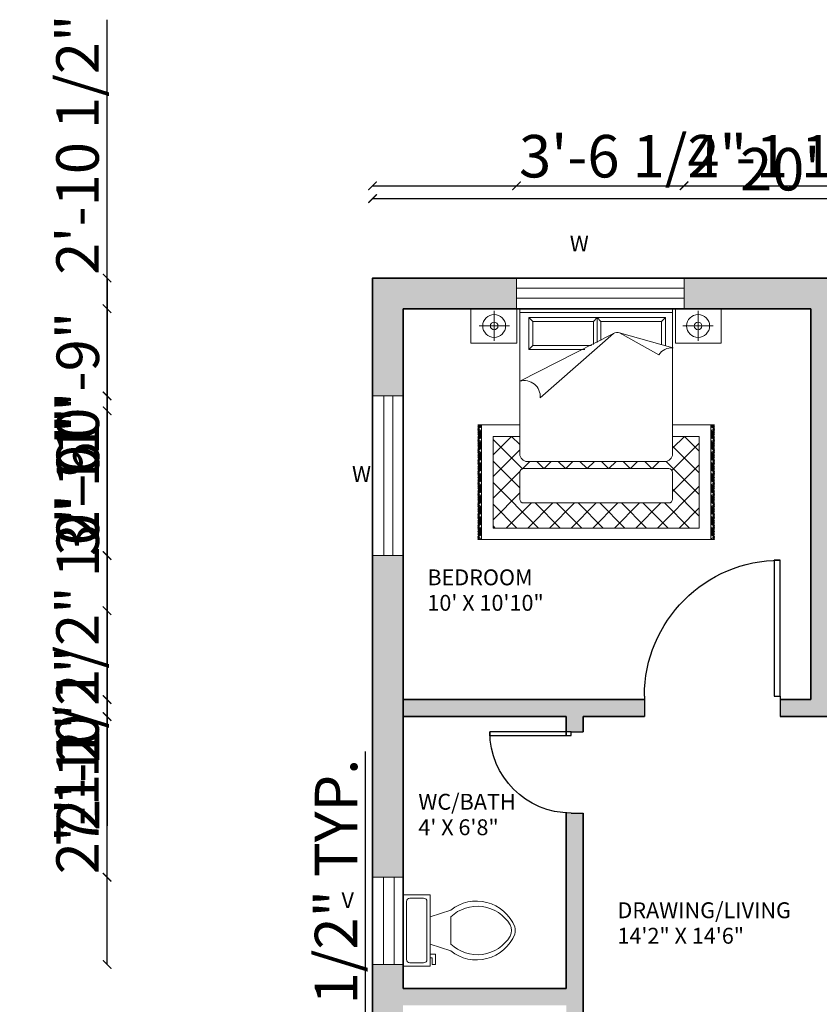
# Model space of a CAD drawing. Units: inches. Extents: x 1750 to 7466, y 1409 to 2004.
# Tile 3 of 5: x 1750 to 1986, y 1715 to 2004. Entities that reach past the tile are written whole.
import ezdxf

# ---------------------------------------------------------------- set-up
doc = ezdxf.new("R2010")
doc.units = ezdxf.units.IN
for name, color, linetype, lineweight in [('A-ANNO-DIMS', 2, 'Continuous', 18), ('A-ANNO-TEXT', 7, 'Continuous', 18), ('A-AREA-IDEN', 7, 'Continuous', 18), ('A-DOOR', 3, 'Continuous', 25), ('A-FLOR-FIXT', 9, 'Continuous', 18), ('A-WALL', 7, 'Continuous', 35), ('BEDS', 15, 'Continuous', 18), ('WINDOW', 4, 'Continuous', 18)]:
    doc.layers.add(name, color=color, linetype=linetype, lineweight=lineweight)
doc.layers.add('A-WALL-PATT', color=18, linetype='Continuous', lineweight=13, true_color=0x000000)
doc.styles.get("Standard").update_dxf_attribs({"font": 'arial.ttf'})
doc.dimstyles.new('ISO-25', dxfattribs={"dimtxt": 12.5, "dimasz": 2.5, "dimexe": 1.25, "dimexo": 0.625, "dimtad": 1, "dimdec": 0, "dimlunit": 4, "dimtxsty": 'Standard', "dimblk": 'ARCHTICK', "dimcen": 2.5, "dimse1": 1, "dimse2": 1, "dimclrd": 2, "dimadec": 0, "dimazin": 0, "dimtfac": 1, "dimtdec": 0, "dimtmove": 0, "dimatfit": 3, "dimfxl": 1, "dimarcsym": 0})

# ---------------------------------------------------------------- blocks, each defined once
blk = doc.blocks.new('A$C4CB008C5')
for p, q in [((0, 3.019), (0.6, 3.019)), ((0, 2.569), (0, 3.019)), ((0.304, 2.6), (0.304, 2.992)), ((0.6, 3.019), (0.6, 2.569)), ((0.64, 1.121), (0.64, 3.021)), ((0.64, 3.021), (2.64, 3.021)), ((0.64, 2.971), (2.64, 2.971)), ((2.64, 3.021), (2.64, 1.121)), ((3.279, 3.019), (2.679, 3.019)), ((2.679, 3.019), (2.679, 2.569)), ((2.975, 2.6), (2.975, 2.992)), ((3.279, 2.569), (3.279, 3.019)), ((0.759, 2.905), (2.547, 2.905)), ((0.759, 2.489), (0.759, 2.905)), ((0.759, 2.905), (0.809, 2.855)), ((0.809, 2.855), (1.603, 2.855)), ((0.809, 2.539), (0.809, 2.855)), ((1.603, 2.855), (1.653, 2.905)), ((1.603, 2.855), (1.603, 2.551)), ((1.653, 2.905), (1.653, 2.579)), ((1.653, 2.905), (1.703, 2.855)), ((1.703, 2.855), (1.703, 2.607)), ((1.703, 2.855), (2.497, 2.855)), ((2.497, 2.855), (2.547, 2.905)), ((2.497, 2.855), (2.497, 2.556)), ((2.547, 2.905), (2.547, 2.54)), ((0.106, 2.796), (0.503, 2.796)), ((3.174, 2.796), (2.776, 2.796)), ((0.64, 2.071), (1.866, 2.698)), ((0.906, 1.854), (1.866, 2.698)), ((1.946, 2.705), (2.646, 2.507)), ((1.946, 2.705), (2.46, 2.418)), ((0.6, 2.569), (0, 2.569)), ((0.809, 2.539), (0.759, 2.489)), ((1.49, 2.489), (0.759, 2.489)), ((1.58, 2.539), (0.809, 2.539)), ((2.679, 2.569), (3.279, 2.569)), ((0.907, 1.867), (0.919, 1.867)), ((0.09, 1.5), (0.64, 1.5)), ((0.09, 1.491), (0.099, 1.5)), ((0.09, 1.473), (0.116, 1.5)), ((0.09, 1.456), (0.134, 1.5)), ((0.09, 1.474), (0.09, 1.475)), ((0.09, 1.438), (0.126, 1.474)), ((0.117, 1.43), (0.09, 1.457)), ((0.14, 1.389), (0.09, 1.439)), ((0.09, 1.42), (0.099, 1.43)), ((0.14, 1.372), (0.09, 1.422)), ((0.14, 1.46), (0.108, 1.492)), ((0.117, 1.412), (0.14, 1.435)), ((0.14, 1.478), (0.118, 1.5)), ((0.14, 1.496), (0.135, 1.5)), ((0.14, 1.442), (0.135, 1.448)), ((0.14, 0), (0.14, 1.5)), ((2.64, 1.5), (3.19, 1.5)), ((3.14, 1.496), (3.144, 1.5)), ((3.14, 1.478), (3.162, 1.5)), ((3.14, 1.5), (3.14, 0)), ((3.14, 1.46), (3.171, 1.492)), ((3.14, 1.442), (3.145, 1.448)), ((3.14, 1.389), (3.19, 1.439)), ((3.162, 1.412), (3.14, 1.435)), ((3.14, 1.372), (3.19, 1.422)), ((3.19, 1.456), (3.145, 1.5)), ((3.19, 1.438), (3.154, 1.474)), ((3.162, 1.43), (3.19, 1.457)), ((3.19, 1.473), (3.163, 1.5)), ((3.19, 1.42), (3.18, 1.43)), ((3.19, 1.491), (3.181, 1.5)), ((3.189, 1.474), (3.19, 1.475)), ((0.09, 1.368), (0.14, 1.417)), ((0.14, 1.354), (0.09, 1.404)), ((0.09, 1.35), (0.14, 1.4)), ((0.14, 1.336), (0.09, 1.386)), ((0.09, 1.332), (0.14, 1.382)), ((0.09, 1.314), (0.14, 1.364)), ((0.09, 1.297), (0.126, 1.333)), ((0.09, 1.333), (0.09, 1.333)), ((0.117, 1.288), (0.09, 1.316)), ((0.14, 1.248), (0.09, 1.298)), ((0.14, 1.319), (0.108, 1.35)), ((0.117, 1.271), (0.14, 1.294)), ((0.14, 1.301), (0.135, 1.306)), ((0.29, 1.108), (0.532, 1.35)), ((0.29, 0.15), (0.29, 1.35)), ((0.29, 1.35), (0.64, 1.35)), ((0.674, 0.926), (0.29, 1.31)), ((0.64, 1.243), (0.533, 1.35)), ((2.64, 1.195), (2.795, 1.35)), ((2.64, 1.35), (2.99, 1.35)), ((2.99, 1.156), (2.795, 1.35)), ((2.99, 1.35), (2.99, 0.15)), ((3.189, 1.368), (3.14, 1.417)), ((3.14, 1.354), (3.19, 1.404)), ((3.19, 1.35), (3.14, 1.4)), ((3.14, 1.336), (3.19, 1.386)), ((3.19, 1.332), (3.14, 1.382)), ((3.19, 1.314), (3.14, 1.364)), ((3.14, 1.319), (3.171, 1.35)), ((3.14, 1.301), (3.145, 1.306)), ((3.14, 1.248), (3.19, 1.298)), ((3.162, 1.271), (3.14, 1.294)), ((3.19, 1.297), (3.154, 1.333)), ((3.162, 1.288), (3.19, 1.316)), ((3.189, 1.333), (3.19, 1.333)), ((0.09, 1.279), (0.099, 1.288)), ((0.14, 1.23), (0.09, 1.28)), ((0.09, 1.227), (0.14, 1.276)), ((0.14, 1.213), (0.09, 1.263)), ((0.09, 1.208), (0.14, 1.258)), ((0.14, 1.195), (0.09, 1.245)), ((0.09, 1.19), (0.14, 1.24)), ((0.09, 1.173), (0.14, 1.223)), ((0.09, 1.191), (0.09, 1.192)), ((0.09, 1.155), (0.126, 1.191)), ((0.117, 1.147), (0.09, 1.174)), ((0.14, 1.177), (0.108, 1.209)), ((0.14, 1.16), (0.135, 1.165)), ((0.29, 0.825), (0.64, 1.175)), ((2.632, 0.904), (2.99, 1.262)), ((2.99, 0.873), (2.64, 1.223)), ((3.14, 1.23), (3.19, 1.28)), ((3.189, 1.227), (3.14, 1.276)), ((3.14, 1.213), (3.19, 1.263)), ((3.19, 1.208), (3.14, 1.258)), ((3.14, 1.195), (3.19, 1.245)), ((3.19, 1.19), (3.14, 1.24)), ((3.19, 1.173), (3.14, 1.223)), ((3.14, 1.177), (3.171, 1.209)), ((3.14, 1.16), (3.145, 1.165)), ((3.19, 1.155), (3.154, 1.191)), ((3.162, 1.147), (3.19, 1.174)), ((3.19, 1.279), (3.18, 1.288)), ((3.189, 1.191), (3.19, 1.192)), ((0.14, 1.107), (0.09, 1.157)), ((0.09, 1.137), (0.099, 1.147)), ((0.14, 1.089), (0.09, 1.139)), ((0.09, 1.085), (0.14, 1.134)), ((0.14, 1.071), (0.09, 1.121)), ((0.09, 1.067), (0.14, 1.117)), ((0.14, 1.054), (0.09, 1.104)), ((0.09, 1.049), (0.14, 1.099)), ((0.09, 1.031), (0.14, 1.081)), ((0.09, 1.05), (0.09, 1.051)), ((0.09, 1.014), (0.126, 1.05)), ((0.117, 1.006), (0.09, 1.033)), ((0.14, 1.036), (0.108, 1.067)), ((0.117, 1.129), (0.14, 1.152)), ((3.14, 1.107), (3.19, 1.157)), ((3.162, 1.129), (3.14, 1.152)), ((3.14, 1.089), (3.19, 1.139)), ((3.189, 1.085), (3.14, 1.134)), ((3.14, 1.071), (3.19, 1.121)), ((3.19, 1.067), (3.14, 1.117)), ((3.14, 1.054), (3.19, 1.104)), ((3.19, 1.049), (3.14, 1.099)), ((3.19, 1.031), (3.14, 1.081)), ((3.14, 1.036), (3.171, 1.067)), ((3.19, 1.014), (3.154, 1.05)), ((3.162, 1.006), (3.19, 1.033)), ((3.19, 1.137), (3.18, 1.147)), ((3.189, 1.05), (3.19, 1.051)), ((0.14, 0.965), (0.09, 1.015)), ((0.09, 0.996), (0.099, 1.006)), ((0.14, 0.948), (0.09, 0.998)), ((0.09, 0.944), (0.14, 0.993)), ((0.14, 0.93), (0.09, 0.98)), ((0.09, 0.925), (0.14, 0.975)), ((0.14, 0.912), (0.09, 0.962)), ((0.09, 0.908), (0.14, 0.958)), ((0.09, 0.89), (0.14, 0.94)), ((0.09, 0.908), (0.09, 0.909)), ((0.09, 0.872), (0.126, 0.908)), ((0.14, 0.894), (0.108, 0.926)), ((0.117, 0.988), (0.14, 1.011)), ((0.14, 1.018), (0.135, 1.023)), ((0.64, 0.677), (0.29, 1.027)), ((0.673, 0.925), (0.769, 1.021)), ((0.69, 0.928), (2.59, 0.928)), ((2.54, 1.021), (0.74, 1.021)), ((0.955, 0.928), (0.861, 1.021)), ((0.959, 0.928), (1.052, 1.021)), ((1.238, 0.928), (1.144, 1.021)), ((1.241, 0.928), (1.335, 1.021)), ((1.52, 0.928), (1.427, 1.021)), ((1.524, 0.928), (1.618, 1.021)), ((1.803, 0.928), (1.71, 1.021)), ((1.807, 0.928), (1.9, 1.021)), ((2.086, 0.928), (1.993, 1.021)), ((2.09, 0.928), (2.183, 1.021)), ((2.369, 0.928), (2.276, 1.021)), ((2.373, 0.928), (2.466, 1.021)), ((2.99, 0.59), (2.557, 1.023)), ((2.64, 0.629), (2.99, 0.979)), ((3.14, 1.018), (3.145, 1.023)), ((3.14, 0.965), (3.19, 1.015)), ((3.162, 0.988), (3.14, 1.011)), ((3.14, 0.948), (3.19, 0.998)), ((3.189, 0.944), (3.14, 0.993)), ((3.14, 0.93), (3.19, 0.98)), ((3.19, 0.925), (3.14, 0.975)), ((3.14, 0.912), (3.19, 0.962)), ((3.19, 0.908), (3.14, 0.958)), ((3.19, 0.89), (3.14, 0.94)), ((3.14, 0.894), (3.171, 0.926)), ((3.19, 0.872), (3.154, 0.908)), ((3.19, 0.996), (3.18, 1.006)), ((3.189, 0.908), (3.19, 0.909)), ((0.117, 0.864), (0.09, 0.891)), ((0.14, 0.824), (0.09, 0.874)), ((0.09, 0.855), (0.099, 0.864)), ((0.14, 0.806), (0.09, 0.856)), ((0.09, 0.802), (0.14, 0.852)), ((0.14, 0.788), (0.09, 0.838)), ((0.09, 0.784), (0.14, 0.834)), ((0.14, 0.771), (0.09, 0.821)), ((0.09, 0.766), (0.14, 0.816)), ((0.09, 0.749), (0.14, 0.799)), ((0.14, 0.753), (0.108, 0.785)), ((0.117, 0.847), (0.14, 0.869)), ((0.14, 0.877), (0.135, 0.882)), ((0.29, 0.542), (0.643, 0.895)), ((0.64, 0.878), (0.64, 0.528)), ((2.64, 0.878), (2.64, 0.528)), ((3.14, 0.877), (3.145, 0.882)), ((3.14, 0.824), (3.19, 0.874)), ((3.162, 0.847), (3.14, 0.869)), ((3.14, 0.806), (3.19, 0.856)), ((3.189, 0.802), (3.14, 0.852)), ((3.14, 0.788), (3.19, 0.838)), ((3.19, 0.784), (3.14, 0.834)), ((3.14, 0.771), (3.19, 0.821)), ((3.19, 0.766), (3.14, 0.816)), ((3.19, 0.749), (3.14, 0.799)), ((3.14, 0.753), (3.171, 0.785)), ((3.162, 0.864), (3.19, 0.891)), ((3.19, 0.855), (3.18, 0.864)), ((0.09, 0.767), (0.09, 0.768)), ((0.09, 0.731), (0.126, 0.767)), ((0.117, 0.723), (0.09, 0.75)), ((0.14, 0.682), (0.09, 0.732)), ((0.09, 0.713), (0.099, 0.723)), ((0.14, 0.665), (0.09, 0.715)), ((0.09, 0.661), (0.14, 0.71)), ((0.14, 0.647), (0.09, 0.697)), ((0.09, 0.642), (0.14, 0.692)), ((0.14, 0.629), (0.09, 0.679)), ((0.09, 0.625), (0.14, 0.675)), ((0.09, 0.607), (0.14, 0.657)), ((0.117, 0.705), (0.14, 0.728)), ((0.14, 0.735), (0.135, 0.74)), ((0.884, 0.15), (0.29, 0.744)), ((2.443, 0.15), (2.99, 0.696)), ((2.99, 0.307), (2.64, 0.657)), ((3.14, 0.735), (3.145, 0.74)), ((3.14, 0.682), (3.19, 0.732)), ((3.162, 0.705), (3.14, 0.728)), ((3.14, 0.665), (3.19, 0.715)), ((3.189, 0.661), (3.14, 0.71)), ((3.14, 0.647), (3.19, 0.697)), ((3.19, 0.642), (3.14, 0.692)), ((3.14, 0.629), (3.19, 0.679)), ((3.19, 0.625), (3.14, 0.675)), ((3.19, 0.607), (3.14, 0.657)), ((3.19, 0.731), (3.154, 0.767)), ((3.162, 0.723), (3.19, 0.75)), ((3.19, 0.713), (3.18, 0.723)), ((3.189, 0.767), (3.19, 0.768)), ((0.09, 0.589), (0.126, 0.626)), ((0.09, 0.626), (0.09, 0.626)), ((0.117, 0.581), (0.09, 0.609)), ((0.14, 0.541), (0.09, 0.591)), ((0.09, 0.572), (0.099, 0.581)), ((0.14, 0.523), (0.09, 0.573)), ((0.09, 0.519), (0.14, 0.569)), ((0.14, 0.506), (0.09, 0.556)), ((0.09, 0.501), (0.14, 0.551)), ((0.14, 0.488), (0.09, 0.538)), ((0.09, 0.483), (0.14, 0.533)), ((0.09, 0.466), (0.14, 0.516)), ((0.14, 0.612), (0.108, 0.643)), ((0.117, 0.564), (0.14, 0.586)), ((0.14, 0.594), (0.135, 0.599)), ((0.29, 0.259), (0.64, 0.609)), ((3.14, 0.612), (3.171, 0.643)), ((3.14, 0.594), (3.145, 0.599)), ((3.14, 0.541), (3.19, 0.591)), ((3.162, 0.564), (3.14, 0.586)), ((3.14, 0.523), (3.19, 0.573)), ((3.189, 0.519), (3.14, 0.569)), ((3.14, 0.506), (3.19, 0.556)), ((3.19, 0.501), (3.14, 0.551)), ((3.14, 0.488), (3.19, 0.538)), ((3.19, 0.483), (3.14, 0.533)), ((3.19, 0.466), (3.14, 0.516)), ((3.19, 0.589), (3.154, 0.626)), ((3.162, 0.581), (3.19, 0.609)), ((3.19, 0.572), (3.18, 0.581)), ((3.189, 0.626), (3.19, 0.626)), ((0.09, 0.484), (0.09, 0.485)), ((0.09, 0.448), (0.126, 0.484)), ((0.117, 0.44), (0.09, 0.467)), ((0.14, 0.399), (0.09, 0.449)), ((0.09, 0.43), (0.099, 0.44)), ((0.14, 0.382), (0.09, 0.432)), ((0.09, 0.378), (0.14, 0.427)), ((0.14, 0.364), (0.09, 0.414)), ((0.09, 0.36), (0.14, 0.41)), ((0.14, 0.346), (0.09, 0.396)), ((0.09, 0.342), (0.14, 0.392)), ((0.14, 0.47), (0.108, 0.502)), ((0.117, 0.422), (0.14, 0.445)), ((0.14, 0.453), (0.135, 0.458)), ((0.601, 0.15), (0.29, 0.462)), ((0.463, 0.15), (0.791, 0.478)), ((0.69, 0.478), (2.59, 0.478)), ((0.746, 0.15), (1.074, 0.478)), ((1.167, 0.15), (0.839, 0.478)), ((1.029, 0.15), (1.357, 0.478)), ((1.45, 0.15), (1.122, 0.478)), ((1.312, 0.15), (1.64, 0.478)), ((1.733, 0.15), (1.405, 0.478)), ((1.595, 0.15), (1.923, 0.478)), ((2.016, 0.15), (1.688, 0.478)), ((1.878, 0.15), (2.206, 0.478)), ((2.298, 0.15), (1.97, 0.478)), ((2.16, 0.15), (2.488, 0.478)), ((2.581, 0.15), (2.253, 0.478)), ((2.864, 0.15), (2.536, 0.478)), ((2.726, 0.15), (2.99, 0.414)), ((3.14, 0.47), (3.171, 0.502)), ((3.14, 0.453), (3.145, 0.458)), ((3.14, 0.399), (3.19, 0.449)), ((3.162, 0.422), (3.14, 0.445)), ((3.14, 0.382), (3.19, 0.432)), ((3.189, 0.378), (3.14, 0.427)), ((3.14, 0.364), (3.19, 0.414)), ((3.19, 0.36), (3.14, 0.41)), ((3.14, 0.346), (3.19, 0.396)), ((3.19, 0.342), (3.14, 0.392)), ((3.19, 0.448), (3.154, 0.484)), ((3.162, 0.44), (3.19, 0.467)), ((3.19, 0.43), (3.18, 0.44)), ((3.189, 0.484), (3.19, 0.485)), ((0.09, 0.324), (0.14, 0.374)), ((0.09, 0.307), (0.126, 0.343)), ((0.09, 0.343), (0.09, 0.343)), ((0.117, 0.299), (0.09, 0.326)), ((0.14, 0.258), (0.09, 0.308)), ((0.09, 0.289), (0.099, 0.299)), ((0.14, 0.24), (0.09, 0.29)), ((0.09, 0.237), (0.14, 0.286)), ((0.14, 0.223), (0.09, 0.273)), ((0.09, 0.218), (0.14, 0.268)), ((0.14, 0.329), (0.108, 0.36)), ((0.117, 0.281), (0.14, 0.304)), ((0.14, 0.311), (0.135, 0.316)), ((3.19, 0.324), (3.14, 0.374)), ((3.14, 0.329), (3.171, 0.36)), ((3.14, 0.311), (3.145, 0.316)), ((3.14, 0.258), (3.19, 0.308)), ((3.162, 0.281), (3.14, 0.304)), ((3.14, 0.24), (3.19, 0.29)), ((3.189, 0.237), (3.14, 0.286)), ((3.14, 0.223), (3.19, 0.273)), ((3.19, 0.218), (3.14, 0.268)), ((3.19, 0.307), (3.154, 0.343)), ((3.162, 0.299), (3.19, 0.326)), ((3.19, 0.289), (3.18, 0.299)), ((3.189, 0.343), (3.19, 0.343)), ((0.14, 0.205), (0.09, 0.255)), ((0.09, 0.201), (0.14, 0.251)), ((0.09, 0.183), (0.14, 0.233)), ((0.09, 0.201), (0.09, 0.202)), ((0.09, 0.165), (0.126, 0.201)), ((0.117, 0.157), (0.09, 0.184)), ((0.14, 0.117), (0.09, 0.167)), ((0.09, 0.148), (0.099, 0.157)), ((0.14, 0.099), (0.09, 0.149)), ((0.09, 0.095), (0.14, 0.144)), ((0.14, 0.081), (0.09, 0.131)), ((0.14, 0.187), (0.108, 0.219)), ((0.117, 0.139), (0.14, 0.162)), ((0.14, 0.17), (0.135, 0.175)), ((0.318, 0.15), (0.29, 0.179)), ((2.99, 0.15), (0.29, 0.15)), ((3.14, 0.205), (3.19, 0.255)), ((3.19, 0.201), (3.14, 0.251)), ((3.19, 0.183), (3.14, 0.233)), ((3.14, 0.187), (3.171, 0.219)), ((3.14, 0.17), (3.145, 0.175)), ((3.14, 0.117), (3.19, 0.167)), ((3.162, 0.139), (3.14, 0.162)), ((3.14, 0.099), (3.19, 0.149)), ((3.189, 0.095), (3.14, 0.144)), ((3.14, 0.081), (3.19, 0.131)), ((3.19, 0.165), (3.154, 0.201)), ((3.162, 0.157), (3.19, 0.184)), ((3.19, 0.148), (3.18, 0.157)), ((3.189, 0.201), (3.19, 0.202)), ((0.09, 0.077), (0.14, 0.127)), ((0.14, 0.064), (0.09, 0.114)), ((0.09, 0.059), (0.14, 0.109)), ((0.09, 0.041), (0.14, 0.091)), ((0.09, 0.06), (0.09, 0.061)), ((0.09, 0.024), (0.126, 0.06)), ((0.117, 0.016), (0.09, 0.043)), ((0.115, 0), (0.09, 0.025)), ((0.09, 0.006), (0.099, 0.016)), ((0.097, 0), (0.09, 0.008)), ((0.14, 0.046), (0.108, 0.078)), ((0.119, 0), (0.14, 0.021)), ((0.14, 0.028), (0.135, 0.033)), ((0.137, 0), (0.14, 0.003)), ((3.19, 0.077), (3.14, 0.127)), ((3.14, 0.064), (3.19, 0.114)), ((3.19, 0.059), (3.14, 0.109)), ((3.19, 0.041), (3.14, 0.091)), ((3.14, 0.046), (3.171, 0.078)), ((3.14, 0.028), (3.145, 0.033)), ((3.16, 0), (3.14, 0.021)), ((3.143, 0), (3.14, 0.003)), ((3.19, 0.024), (3.154, 0.06)), ((3.162, 0.016), (3.19, 0.043)), ((3.164, 0), (3.19, 0.025)), ((3.19, 0.006), (3.18, 0.016)), ((3.182, 0), (3.19, 0.008)), ((3.189, 0.06), (3.19, 0.061)), ((0.09, 0), (3.19, 0))]:
    blk.add_line(p, q)
for centre, radius in [((0.304, 2.796), 0.15), ((0.304, 2.796), 0.05), ((2.975, 2.796), 0.15), ((2.975, 2.796), 0.05)]:
    blk.add_circle(centre, radius)
for centre, radius, start, end in [((1.915, 2.61), 0.1, 71.7215, 119.0799), ((2.626, 2.31), 0.198, 84.1725, 146.9889), ((0.7, 1.873), 0.207, 354.6422, 106.9775), ((0.74, 1.121), 0.1, 180, 270), ((2.54, 1.121), 0.1, 270, 0), ((0.69, 0.878), 0.05, 90, 180), ((2.59, 0.878), 0.05, 0, 90), ((0.69, 0.528), 0.05, 180, 270), ((2.59, 0.528), 0.05, 270, 0)]:
    blk.add_arc(centre, radius, start, end)
blk = doc.blocks.new('*U9')
for p, q in [((9.5, -6), (9.5, -2)), ((-10, -8.5), (-8, -8.5)), ((-10, -9.5), (-10, -8.5)), ((-8, -8.5), (-8, -8)), ((-7, -8), (-7, -9.5)), ((-4, -8), (-6, -14)), ((4, -8), (6, -14)), ((-7, -9.5), (-10, -9.5)), ((4, -14), (-4, -14))]:
    blk.add_line(p, q)
blk.add_lwpolyline([(10.5, -8), (10.5, 0), (-10.5, 0), (-10.5, -8)], close=True)
for points in [[(-9.5, -2), (-9.5, -6)], [(8.5, -1), (-8.5, -1)], [(-8.5, -7), (8.5, -7)]]:
    blk.add_lwpolyline(points)
for centre, radius, start, end in [((-8.62, -1.88), 0.884, 81.8699, 188.1301), ((8.62, -1.88), 0.884, 351.8699, 98.1301), ((-8.62, -6.12), 0.884, 171.8699, 278.1301), ((8.62, -6.12), 0.884, 261.8699, 8.1301), ((3.52, -21.58), 12.17, 141.4691, 247.9714), ((4.2, -21.82), 11.33, 136.3677, 238.9468), ((-3.52, -21.58), 12.17, 292.0284, 38.5307), ((-4.2, -21.82), 11.33, 301.053, 43.6321), ((0, -27.88), 4, 245.7318, 294.2682), ((0, -29), 4, 254.8605, 285.1395)]:
    blk.add_arc(centre, radius, start, end)
blk = doc.blocks.new('*U11')
for p, q in [((0, 0), (0, -6)), ((40, 0), (40, -6))]:
    blk.add_line(p, q)
blk.add_lwpolyline([(0, 0), (0, 40), (1.75, 40), (1.75, 0)], close=True)
blk.add_arc((0, 0), 40, 0, 90)
blk = doc.blocks.new('_ArchTick')
at = {"color": 0, "linetype": 'ByBlock', "const_width": 0.15}
blk.add_lwpolyline([(-0.5, -0.5), (0.5, 0.5)], dxfattribs=at)
blk = doc.blocks.new('*D13')
at = {"layer": 'A-ANNO-DIMS', "color": 0, "lineweight": -2, "transparency": 16777216}
blk.add_line((1854.13, 1951.57), (2094.13, 1951.57), dxfattribs=at)
at = {"layer": 'Defpoints', "color": 0, "transparency": 16777216}
for p in [(2094.13, 1951.57), (1854.13, 1928.17), (2094.13, 1928.17)]:
    blk.add_point(p, dxfattribs=at)
at = {"layer": 'A-ANNO-DIMS', "color": 0, "lineweight": -2, "transparency": 16777216, "xscale": 2.5, "yscale": 2.5, "zscale": 2.5, "rotation": 180}
blk.add_blockref('_ArchTick', (1854.13, 1951.57), dxfattribs=at)
at = {"layer": 'A-ANNO-DIMS', "color": 0, "lineweight": -2, "transparency": 16777216, "xscale": 2.5, "yscale": 2.5, "zscale": 2.5}
blk.add_blockref('_ArchTick', (2094.13, 1951.57), dxfattribs=at)
at = {"layer": 'A-ANNO-DIMS', "color": 0, "transparency": 16777216, "insert": (1974.13, 1958.58), "char_height": 12.5, "attachment_point": 5}
blk.add_mtext("20'", dxfattribs=at)
blk = doc.blocks.new('*D15')
at = {"layer": 'A-ANNO-DIMS', "color": 2, "lineweight": -2, "transparency": 16777216}
for p, q in [((1852.08, 1639.61), (1852.08, 1788.89)), ((1852.08, 1565.91), (1852.08, 1639.61))]:
    blk.add_line(p, q, dxfattribs=at)
at = {"layer": 'Defpoints', "color": 0, "transparency": 16777216}
for p in [(1852.08, 1639.61), (1863.13, 1639.61), (1863.13, 1565.91)]:
    blk.add_point(p, dxfattribs=at)
at = {"layer": 'A-ANNO-DIMS', "color": 2, "lineweight": -2, "transparency": 16777216, "xscale": 2.5, "yscale": 2.5, "zscale": 2.5}
for p, rotation in [((1852.08, 1639.61), 90), ((1852.08, 1565.91), 270)]:
    blk.add_blockref('_ArchTick', p, dxfattribs=dict(at, rotation=rotation))
at = {"layer": 'A-ANNO-DIMS', "color": 0, "transparency": 16777216, "insert": (1844.99, 1715.5), "char_height": 12.5, "attachment_point": 5, "rotation": 90}
blk.add_mtext('BED 6\'-1 1/2" TYP.', dxfattribs=at)
blk = doc.blocks.new('*D34')
at = {"layer": 'A-ANNO-DIMS', "color": 2, "lineweight": -2, "transparency": 16777216}
for p, q in [((1775.98, 1751.88), (1775.98, 1818.19)), ((1775.98, 1726.23), (1775.98, 1751.88))]:
    blk.add_line(p, q, dxfattribs=at)
at = {"layer": 'Defpoints', "color": 0, "transparency": 16777216}
for p in [(1775.98, 1751.88), (1854.13, 1751.88), (1854.13, 1726.23)]:
    blk.add_point(p, dxfattribs=at)
at = {"layer": 'A-ANNO-DIMS', "color": 2, "lineweight": -2, "transparency": 16777216, "xscale": 2.5, "yscale": 2.5, "zscale": 2.5}
for p, rotation in [((1775.98, 1751.88), 90), ((1775.98, 1726.23), 270)]:
    blk.add_blockref('_ArchTick', p, dxfattribs=dict(at, rotation=rotation))
at = {"layer": 'A-ANNO-DIMS', "color": 0, "transparency": 16777216, "insert": (1768.9, 1786.29), "char_height": 12.5, "attachment_point": 5, "rotation": 90}
blk.add_mtext('2\'-1 1/2"', dxfattribs=at)
blk = doc.blocks.new('*D35')
at = {"layer": 'A-ANNO-DIMS', "color": 2, "lineweight": -2, "transparency": 16777216}
blk.add_line((1775.98, 1751.88), (1775.98, 1846.52), dxfattribs=at)
at = {"layer": 'Defpoints', "color": 0, "transparency": 16777216}
for p in [(1775.98, 1846.52), (1854.13, 1846.52), (1854.13, 1751.88)]:
    blk.add_point(p, dxfattribs=at)
at = {"layer": 'A-ANNO-DIMS', "color": 2, "lineweight": -2, "transparency": 16777216, "xscale": 2.5, "yscale": 2.5, "zscale": 2.5}
for p, rotation in [((1775.98, 1846.52), 90), ((1775.98, 1751.88), 270)]:
    blk.add_blockref('_ArchTick', p, dxfattribs=dict(at, rotation=rotation))
at = {"layer": 'A-ANNO-DIMS', "color": 0, "transparency": 16777216, "insert": (1768.9, 1799.2), "char_height": 12.5, "attachment_point": 5, "rotation": 90}
blk.add_mtext('7\'-10 1/2"', dxfattribs=at)
blk = doc.blocks.new('*D36')
at = {"layer": 'A-ANNO-DIMS', "color": 2, "lineweight": -2, "transparency": 16777216}
blk.add_line((1775.98, 1846.52), (1775.98, 1893.52), dxfattribs=at)
at = {"layer": 'Defpoints', "color": 0, "transparency": 16777216}
for p in [(1775.98, 1893.52), (1854.13, 1893.52), (1854.13, 1846.52)]:
    blk.add_point(p, dxfattribs=at)
at = {"layer": 'A-ANNO-DIMS', "color": 2, "lineweight": -2, "transparency": 16777216, "xscale": 2.5, "yscale": 2.5, "zscale": 2.5}
for p, rotation in [((1775.98, 1893.52), 90), ((1775.98, 1846.52), 270)]:
    blk.add_blockref('_ArchTick', p, dxfattribs=dict(at, rotation=rotation))
at = {"layer": 'A-ANNO-DIMS', "color": 0, "transparency": 16777216, "insert": (1768.97, 1870.02), "char_height": 12.5, "attachment_point": 5, "rotation": 90}
blk.add_mtext('3\'-11"', dxfattribs=at)
blk = doc.blocks.new('*D37')
at = {"layer": 'A-ANNO-DIMS', "color": 2, "lineweight": -2, "transparency": 16777216}
for p, q in [((1775.98, 1928.17), (1775.98, 2004.2)), ((1775.98, 1893.52), (1775.98, 1928.17))]:
    blk.add_line(p, q, dxfattribs=at)
at = {"layer": 'Defpoints', "color": 0, "transparency": 16777216}
for p in [(1775.98, 1928.17), (1854.13, 1928.17), (1854.13, 1893.52)]:
    blk.add_point(p, dxfattribs=at)
at = {"layer": 'A-ANNO-DIMS', "color": 2, "lineweight": -2, "transparency": 16777216, "xscale": 2.5, "yscale": 2.5, "zscale": 2.5}
for p, rotation in [((1775.98, 1928.17), 90), ((1775.98, 1893.52), 270)]:
    blk.add_blockref('_ArchTick', p, dxfattribs=dict(at, rotation=rotation))
at = {"layer": 'A-ANNO-DIMS', "color": 0, "transparency": 16777216, "insert": (1768.9, 1967.43), "char_height": 12.5, "attachment_point": 5, "rotation": 90}
blk.add_mtext('2\'-10 1/2"', dxfattribs=at)
blk = doc.blocks.new('*D39')
at = {"layer": 'A-ANNO-DIMS', "color": 2, "lineweight": -2, "transparency": 16777216}
for p, q in [((1775.98, 1919.17), (1775.98, 1889.13)), ((1775.98, 1889.13), (1775.98, 1851.94))]:
    blk.add_line(p, q, dxfattribs=at)
at = {"layer": 'Defpoints', "color": 0, "transparency": 16777216}
for p in [(2024.28, 1919.17), (1775.98, 1889.13), (2024.28, 1889.13)]:
    blk.add_point(p, dxfattribs=at)
at = {"layer": 'A-ANNO-DIMS', "color": 2, "lineweight": -2, "transparency": 16777216, "xscale": 2.5, "yscale": 2.5, "zscale": 2.5}
for p, rotation in [((1775.98, 1919.17), 90), ((1775.98, 1889.13), 270)]:
    blk.add_blockref('_ArchTick', p, dxfattribs=dict(at, rotation=rotation))
at = {"layer": 'A-ANNO-DIMS', "color": 0, "transparency": 16777216, "insert": (1768.98, 1869.28), "char_height": 12.5, "attachment_point": 5, "rotation": 90}
blk.add_mtext('2\'-6"', dxfattribs=at)
blk = doc.blocks.new('*D46')
at = {"layer": 'A-ANNO-DIMS', "color": 2, "lineweight": -2, "transparency": 16777216}
for p, q in [((1775.98, 1830.3), (1775.98, 1804.17)), ((1775.98, 1804.17), (1775.98, 1766.97))]:
    blk.add_line(p, q, dxfattribs=at)
at = {"layer": 'Defpoints', "color": 0, "transparency": 16777216}
for p in [(2066.63, 1830.3), (1775.98, 1804.17), (2059.72, 1804.17)]:
    blk.add_point(p, dxfattribs=at)
at = {"layer": 'A-ANNO-DIMS', "color": 2, "lineweight": -2, "transparency": 16777216, "xscale": 2.5, "yscale": 2.5, "zscale": 2.5}
for p, rotation in [((1775.98, 1830.3), 90), ((1775.98, 1804.17), 270)]:
    blk.add_blockref('_ArchTick', p, dxfattribs=dict(at, rotation=rotation))
at = {"layer": 'A-ANNO-DIMS', "color": 0, "transparency": 16777216, "insert": (1769.08, 1784.32), "char_height": 12.5, "attachment_point": 5, "rotation": 90}
blk.add_mtext('2\'-2"', dxfattribs=at)
blk = doc.blocks.new('*D47')
at = {"layer": 'A-ANNO-DIMS', "color": 2, "lineweight": -2, "transparency": 16777216}
for p, q in [((1775.98, 1928.17), (1775.98, 1919.17)), ((1775.98, 1919.17), (1775.98, 1882.19))]:
    blk.add_line(p, q, dxfattribs=at)
at = {"layer": 'Defpoints', "color": 0, "transparency": 16777216}
for p in [(2022.32, 1928.17), (1775.98, 1919.17), (2022.32, 1919.17)]:
    blk.add_point(p, dxfattribs=at)
at = {"layer": 'A-ANNO-DIMS', "color": 2, "lineweight": -2, "transparency": 16777216, "xscale": 2.5, "yscale": 2.5, "zscale": 2.5}
for p, rotation in [((1775.98, 1928.17), 90), ((1775.98, 1919.17), 270)]:
    blk.add_blockref('_ArchTick', p, dxfattribs=dict(at, rotation=rotation))
at = {"layer": 'A-ANNO-DIMS', "color": 0, "transparency": 16777216, "insert": (1768.98, 1899.43), "char_height": 12.5, "attachment_point": 5, "rotation": 90}
blk.add_mtext('0\'-9"', dxfattribs=at)
blk = doc.blocks.new('*D48')
at = {"layer": 'A-ANNO-DIMS', "color": 2, "lineweight": -2, "transparency": 16777216}
for p, q in [((1983.13, 1421.02), (1988.13, 1421.02)), ((1988.13, 1421.02), (2025.11, 1421.02))]:
    blk.add_line(p, q, dxfattribs=at)
at = {"layer": 'Defpoints', "color": 0, "transparency": 16777216}
for p in [(1983.13, 1804.17), (1988.13, 1804.17), (1988.13, 1421.02)]:
    blk.add_point(p, dxfattribs=at)
at = {"layer": 'A-ANNO-DIMS', "color": 2, "lineweight": -2, "transparency": 16777216, "xscale": 2.5, "yscale": 2.5, "zscale": 2.5, "rotation": 180}
blk.add_blockref('_ArchTick', (1983.13, 1421.02), dxfattribs=at)
at = {"layer": 'A-ANNO-DIMS', "color": 2, "lineweight": -2, "transparency": 16777216, "xscale": 2.5, "yscale": 2.5, "zscale": 2.5}
blk.add_blockref('_ArchTick', (1988.13, 1421.02), dxfattribs=at)
at = {"layer": 'A-ANNO-DIMS', "color": 0, "transparency": 16777216, "insert": (2007.87, 1428.02), "char_height": 12.5, "attachment_point": 5}
blk.add_mtext('0\'-5"', dxfattribs=at)
blk = doc.blocks.new('*D49')
at = {"layer": 'A-ANNO-DIMS', "color": 2, "lineweight": -2, "transparency": 16777216}
for p, q in [((1854.13, 1955.32), (1896.49, 1955.32)), ((1896.49, 1955.32), (1962.58, 1955.32))]:
    blk.add_line(p, q, dxfattribs=at)
at = {"layer": 'Defpoints', "color": 0, "transparency": 16777216}
for p in [(1896.49, 1955.32), (1854.13, 1928.17), (1896.49, 1928.17)]:
    blk.add_point(p, dxfattribs=at)
at = {"layer": 'A-ANNO-DIMS', "color": 2, "lineweight": -2, "transparency": 16777216, "xscale": 2.5, "yscale": 2.5, "zscale": 2.5, "rotation": 180}
blk.add_blockref('_ArchTick', (1854.13, 1955.32), dxfattribs=at)
at = {"layer": 'A-ANNO-DIMS', "color": 2, "lineweight": -2, "transparency": 16777216, "xscale": 2.5, "yscale": 2.5, "zscale": 2.5}
blk.add_blockref('_ArchTick', (1896.49, 1955.32), dxfattribs=at)
at = {"layer": 'A-ANNO-DIMS', "color": 0, "transparency": 16777216, "insert": (1930.79, 1962.41), "char_height": 12.5, "attachment_point": 5}
blk.add_mtext('3\'-6 1/2"', dxfattribs=at)
blk = doc.blocks.new('*D50')
at = {"layer": 'A-ANNO-DIMS', "color": 2, "lineweight": -2, "transparency": 16777216}
for p, q in [((1896.49, 1955.32), (1945.82, 1955.32)), ((1945.82, 1955.32), (2012.43, 1955.32))]:
    blk.add_line(p, q, dxfattribs=at)
at = {"layer": 'Defpoints', "color": 0, "transparency": 16777216}
for p in [(1945.82, 1955.32), (1896.49, 1928.17), (1945.82, 1928.17)]:
    blk.add_point(p, dxfattribs=at)
at = {"layer": 'A-ANNO-DIMS', "color": 2, "lineweight": -2, "transparency": 16777216, "xscale": 2.5, "yscale": 2.5, "zscale": 2.5, "rotation": 180}
blk.add_blockref('_ArchTick', (1896.49, 1955.32), dxfattribs=at)
at = {"layer": 'A-ANNO-DIMS', "color": 2, "lineweight": -2, "transparency": 16777216, "xscale": 2.5, "yscale": 2.5, "zscale": 2.5}
blk.add_blockref('_ArchTick', (1945.82, 1955.32), dxfattribs=at)
at = {"layer": 'A-ANNO-DIMS', "color": 0, "transparency": 16777216, "insert": (1980.37, 1962.4), "char_height": 12.5, "attachment_point": 5}
blk.add_mtext('4\'-1 1/2"', dxfattribs=at)
blk = doc.blocks.new('*D55')
at = {"layer": 'A-ANNO-DIMS', "color": 2, "lineweight": -2, "transparency": 16777216}
blk.add_line((1775.98, 1928.17), (1775.98, 1799.17), dxfattribs=at)
at = {"layer": 'Defpoints', "color": 0, "transparency": 16777216}
for p in [(2022.32, 1928.17), (1775.98, 1799.17), (1995.93, 1799.17)]:
    blk.add_point(p, dxfattribs=at)
at = {"layer": 'A-ANNO-DIMS', "color": 2, "lineweight": -2, "transparency": 16777216, "xscale": 2.5, "yscale": 2.5, "zscale": 2.5}
for p, rotation in [((1775.98, 1928.17), 90), ((1775.98, 1799.17), 270)]:
    blk.add_blockref('_ArchTick', p, dxfattribs=dict(at, rotation=rotation))
at = {"layer": 'A-ANNO-DIMS', "color": 0, "transparency": 16777216, "insert": (1768.98, 1863.67), "char_height": 12.5, "attachment_point": 5, "rotation": 90}
blk.add_mtext('10\'-9"', dxfattribs=at)

msp = doc.modelspace()

# ---------------------------------------------------------------- hatches: boundary and pattern name
at = {"layer": 'A-WALL-PATT'}
h = msp.add_hatch(color=256, dxfattribs=at)
h.dxf.hatch_style = 1
h.paths.add_polyline_path([(1896.49, 1928.17), (1854.13, 1928.17), (1854.13, 1893.52), (1863.13, 1893.52), (1863.13, 1919.17), (1896.49, 1919.17)])
h.paths.add_polyline_path([(2022.32, 1928.17), (1945.82, 1928.17), (1945.82, 1919.17), (1983.13, 1919.17), (1983.13, 1804.17), (1974.13, 1804.17), (1974.13, 1799.17), (1995.93, 1799.17), (1995.93, 1804.17), (1988.13, 1804.17), (1988.13, 1919.17), (2022.32, 1919.17)])
h.paths.add_polyline_path([(2094.13, 1928.17), (2070.34, 1928.17), (2070.34, 1919.17), (2085.13, 1919.17), (2085.13, 1875.24), (2094.13, 1875.24)])
h.paths.add_polyline_path([(2094.13, 1827.64), (2085.13, 1827.64), (2085.13, 1804.17), (2035.93, 1804.17), (2035.93, 1799.17), (2085.13, 1799.17), (2085.13, 1763.18), (2094.13, 1763.18)])
h.paths.add_polyline_path([(1863.13, 1846.52), (1854.13, 1846.52), (1854.13, 1751.88), (1863.13, 1751.88)])
h.paths.add_polyline_path([(1934.13, 1804.17), (1863.13, 1804.17), (1863.13, 1799.17), (1911.13, 1799.17), (1911.13, 1794.68), (1912.55, 1794.68), (1916.13, 1794.68), (1916.13, 1799.17), (1934.13, 1799.17)])
h.paths.add_polyline_path([(1863.13, 1726.23), (1854.13, 1726.23), (1854.13, 1709.82), (1863.13, 1709.82), (1863.13, 1714.17), (1911.13, 1714.17), (1911.13, 1671.17), (1887.9, 1671.17, -0.01479), (1887.95, 1669.75), (1887.95, 1666.17), (1916.13, 1666.17), (1940.64, 1666.17), (1940.64, 1671.17), (1916.13, 1671.17), (1916.13, 1770.77), (1912.55, 1770.77, -0.01479), (1911.13, 1770.81), (1911.13, 1719.17), (1863.13, 1719.17)])
h.paths.add_polyline_path([(1863.13, 1684.17), (1854.13, 1684.17), (1854.13, 1625.24), (1863.13, 1625.24)])
h.paths.add_polyline_path([(1863.13, 1577.33), (1854.13, 1577.33), (1854.13, 1526.31), (1863.13, 1526.31), (1863.13, 1544.17), (1983.13, 1544.17), (1988.13, 1544.17), (1990.13, 1544.17), (1990.13, 1549.17), (1990.13, 1620.17), (1996.77, 1620.17), (1996.77, 1625.17), (1990.13, 1625.17), (1990.13, 1666.17), (1990.13, 1671.17), (1980.64, 1671.17), (1980.64, 1666.17), (1985.13, 1666.17), (1985.13, 1625.17), (1985.13, 1549.17), (1863.13, 1549.17)])
h.paths.add_polyline_path([(1988.13, 1457.17), (1863.13, 1457.17), (1863.13, 1497.36), (1854.13, 1497.36), (1854.13, 1448.17), (1988.13, 1448.17)])
h.paths.add_polyline_path([(2031.23, 1454.78), (1988.13, 1454.78), (1988.13, 1450.91), (2031.23, 1450.91)])
h.paths.add_polyline_path([(2074.33, 1454.78), (2037.79, 1454.78), (2037.79, 1450.91), (2074.33, 1450.91)], flags=17)
h.paths.add_polyline_path([(2094.13, 1714.84), (2085.13, 1714.84), (2085.13, 1625.17), (2036.77, 1625.17), (2036.77, 1620.17), (2085.13, 1620.17), (2085.13, 1457.17), (2074.33, 1457.17), (2074.33, 1448.17), (2094.13, 1448.17)])
h.paths.add_polyline_path([(1846.92, 1867), (1855.4, 1867), (1855.4, 1874), (1846.92, 1874)], flags=9)
h.paths.add_polyline_path([(1885.75, 1686.15), (1909.97, 1686.15), (1909.97, 1693.31), (1885.75, 1693.31)], flags=25)
h.paths.add_polyline_path([(1885.73, 1693.64), (1900.82, 1693.64), (1900.82, 1700.88), (1885.73, 1700.88)], flags=25)
h.paths.add_polyline_path([(1866.42, 1762.99), (1892.45, 1762.99), (1892.45, 1770.14), (1866.42, 1770.14)], flags=25)
h.paths.add_polyline_path([(1866.4, 1770.47), (1898.87, 1770.47), (1898.87, 1777.71), (1866.4, 1777.71)], flags=9)
h.paths.add_polyline_path([(1925.02, 1731.07), (1964.24, 1731.07), (1964.24, 1738.22), (1925.02, 1738.22)], flags=9)
h.paths.add_polyline_path([(1925.01, 1738.55), (1982.11, 1738.55), (1982.11, 1745.79), (1925.01, 1745.79)], flags=9)
h.paths.add_polyline_path([(1995.48, 1862.99), (2034.71, 1862.99), (2034.71, 1870.14), (1995.48, 1870.14)], flags=9)
h.paths.add_polyline_path([(1995.47, 1870.47), (2026.49, 1870.47), (2026.49, 1877.71), (1995.47, 1877.71)], flags=9)
h.paths.add_polyline_path([(1869.07, 1829.02), (1905.98, 1829.02), (1905.98, 1836.17), (1869.07, 1836.17)], flags=9)
h.paths.add_polyline_path([(1869.05, 1836.5), (1905.15, 1836.5), (1905.15, 1843.74), (1869.05, 1843.74)], flags=9)

# ---------------------------------------------------------------- linework, layer by layer
at = {"layer": 'A-WALL'}
for p, q in [((1863.13, 1919.17), (1983.13, 1919.17)), ((1863.13, 1719.17), (1863.13, 1919.17)), ((1983.13, 1804.17), (1983.13, 1919.17)), ((1863.13, 1804.17), (1934.13, 1804.17)), ((1974.13, 1804.17), (1983.13, 1804.17)), ((1863.13, 1799.17), (1911.13, 1799.17)), ((1911.13, 1793.64), (1911.13, 1799.17)), ((1916.13, 1794.68), (1916.13, 1799.17)), ((1916.13, 1799.17), (1934.13, 1799.17)), ((1974.13, 1799.17), (1995.93, 1799.17)), ((1911.13, 1719.17), (1911.13, 1770.81)), ((1916.13, 1671.17), (1916.13, 1770.77)), ((1863.13, 1719.17), (1911.13, 1719.17))]:
    msp.add_line(p, q, dxfattribs=at)
msp.add_lwpolyline([(1988.13, 1448.17), (1854.13, 1448.17), (1854.13, 1928.17), (2094.13, 1928.17), (2094.13, 1448.17), (2074.33, 1448.17)], dxfattribs=at)
at = {"layer": 'WINDOW'}
for p, q in [((1896.49, 1928.17), (1896.49, 1919.17)), ((1945.82, 1928.17), (1896.49, 1928.17)), ((1945.82, 1919.17), (1945.82, 1928.17)), ((1945.82, 1925.25), (1896.49, 1925.25)), ((1945.82, 1922.29), (1896.49, 1922.29)), ((1896.49, 1919.17), (1945.82, 1919.17)), ((1863.13, 1893.52), (1854.13, 1893.52)), ((1854.13, 1893.52), (1854.13, 1846.52)), ((1857.44, 1893.52), (1857.44, 1846.52)), ((1860.14, 1893.52), (1860.14, 1846.52)), ((1863.13, 1846.52), (1863.13, 1893.52)), ((1854.13, 1846.52), (1863.13, 1846.52)), ((1863.13, 1751.88), (1854.13, 1751.88)), ((1854.13, 1751.88), (1854.13, 1726.23)), ((1857.37, 1751.88), (1857.37, 1726.23)), ((1860.47, 1751.88), (1860.47, 1726.23)), ((1863.13, 1726.23), (1863.13, 1751.88)), ((1854.13, 1726.23), (1863.13, 1726.23))]:
    msp.add_line(p, q, dxfattribs=at)

# ---------------------------------------------------------------- block references
at = {"layer": 'A-DOOR', "xscale": -1}
msp.add_blockref('*U11', (1974.13, 1805.17), dxfattribs=at)
at = {"layer": 'A-DOOR', "xscale": -0.5977371973788693, "yscale": 0.5977371973788693, "zscale": 0.5977371973788693, "rotation": 90}
msp.add_blockref('*U11', (1912.55, 1794.68), dxfattribs=at)
at = {"layer": 'A-FLOR-FIXT', "rotation": 90}
msp.add_blockref('*U9', (1863.13, 1736.22), dxfattribs=at)
at = {"layer": 'BEDS', "xscale": 22.47616773198522, "yscale": 22.47616773198522, "zscale": 22.47616773198522}
msp.add_blockref('A$C4CB008C5', (1883.09, 1851.26), dxfattribs=at)

# ---------------------------------------------------------------- texts
at = {"layer": 'A-ANNO-TEXT'}
for s, p in [('W', (1912.18, 1936)), ('W', (1848.08, 1868.17)), ('V', (1844.98, 1742.79))]:
    msp.add_text(s, height=4.67, dxfattribs=at).set_placement(p)
at = {"layer": 'A-AREA-IDEN'}
for s, height, p in [('BEDROOM', 4.666, (1870.26, 1837.79)), ('10\' X 10\'10"', 4.6662, (1870.26, 1830.29)), ('WC/BATH', 4.666, (1867.61, 1771.76)), ('4\' X 6\'8"', 4.666, (1867.61, 1764.26)), ('DRAWING/LIVING', 4.6662, (1926.21, 1739.84)), ('14\'2" X 14\'6"', 4.6662, (1926.21, 1732.34))]:
    msp.add_text(s, height=height, dxfattribs=at).set_placement(p)

# ---------------------------------------------------------------- dimensions: what is measured, and where the dimension line sits
at = {"layer": 'A-ANNO-DIMS'}
for base, p1, p2, picture, middle in [((1775.9834, 1928.1652), (1854.1334, 1893.5191), (1854.1334, 1928.1652), '*D37', (1768.8952, 1967.4302)), ((1775.98, 1919.17), (2022.32, 1928.17), (2022.32, 1919.17), '*D47', (1768.98, 1899.43)), ((1775.98, 1799.17), (2022.32, 1928.17), (1995.93, 1799.17), '*D55', (1768.98, 1863.67)), ((1775.98, 1889.13), (2024.28, 1919.17), (2024.28, 1889.13), '*D39', (1768.98, 1869.28)), ((1775.98, 1893.52), (1854.13, 1846.52), (1854.13, 1893.52), '*D36', (1768.97, 1870.02)), ((1775.98, 1846.52), (1854.13, 1751.88), (1854.13, 1846.52), '*D35', (1768.9, 1799.2)), ((1775.98, 1804.17), (2066.63, 1830.3), (2059.72, 1804.17), '*D46', (1769.08, 1784.32)), ((1775.9834, 1751.8767), (1854.1334, 1726.2312), (1854.1334, 1751.8767), '*D34', (1768.8952, 1786.2858))]:
    dim = msp.add_linear_dim(base=base, p1=p1, p2=p2, angle=90, dimstyle='ISO-25', override={"dimdec": 1, "dimlfac": 1, "dimrnd": 0, "dimzin": 1, "dimdsep": 46, "dimlunit": 4, "dimfrac": 2}, dxfattribs=at)
    dim.commit()
    dim.dimension.update_dxf_attribs({"geometry": picture, "text_midpoint": middle})
for base, p1, p2, override, picture, middle in [((1896.49, 1955.32), (1854.13, 1928.17), (1896.49, 1928.17), {"dimdec": 1, "dimlfac": 1, "dimrnd": 0, "dimzin": 1, "dimdsep": 46, "dimlunit": 4, "dimfrac": 2}, '*D49', (1930.79, 1962.41)), ((1945.82, 1955.32), (1896.49, 1928.17), (1945.82, 1928.17), {"dimdec": 1, "dimlfac": 1, "dimrnd": 0, "dimzin": 1, "dimdsep": 46, "dimlunit": 4, "dimfrac": 2}, '*D50', (1980.37, 1962.4)), ((2094.13, 1951.57), (1854.13, 1928.17), (2094.13, 1928.17), {"dimclrd": 0, "dimclre": 0, "dimclrt": 0}, '*D13', (1974.13, 1958.58)), ((1988.13, 1421.02), (1983.13, 1804.17), (1988.13, 1804.17), {"dimdec": 1, "dimlfac": 1, "dimrnd": 0, "dimzin": 1, "dimdsep": 46, "dimlunit": 4, "dimfrac": 2}, '*D48', (2007.87, 1428.02))]:
    dim = msp.add_linear_dim(base=base, p1=p1, p2=p2, dimstyle='ISO-25', override=override, dxfattribs=at)
    dim.commit()
    dim.dimension.update_dxf_attribs({"geometry": picture, "text_midpoint": middle})
dim = msp.add_linear_dim(base=(1852.08, 1639.61), p1=(1863.13, 1565.91), p2=(1863.13, 1639.61), angle=90, text='BED <> TYP.', dimstyle='ISO-25', override={"dimdec": 1, "dimlfac": 1, "dimrnd": 0, "dimzin": 1, "dimdsep": 46, "dimlunit": 4, "dimfrac": 2}, dxfattribs=at)
dim.commit()
dim.dimension.update_dxf_attribs({"geometry": '*D15', "text_midpoint": (1844.99, 1715.5)})

doc.saveas('drawing.dxf')
